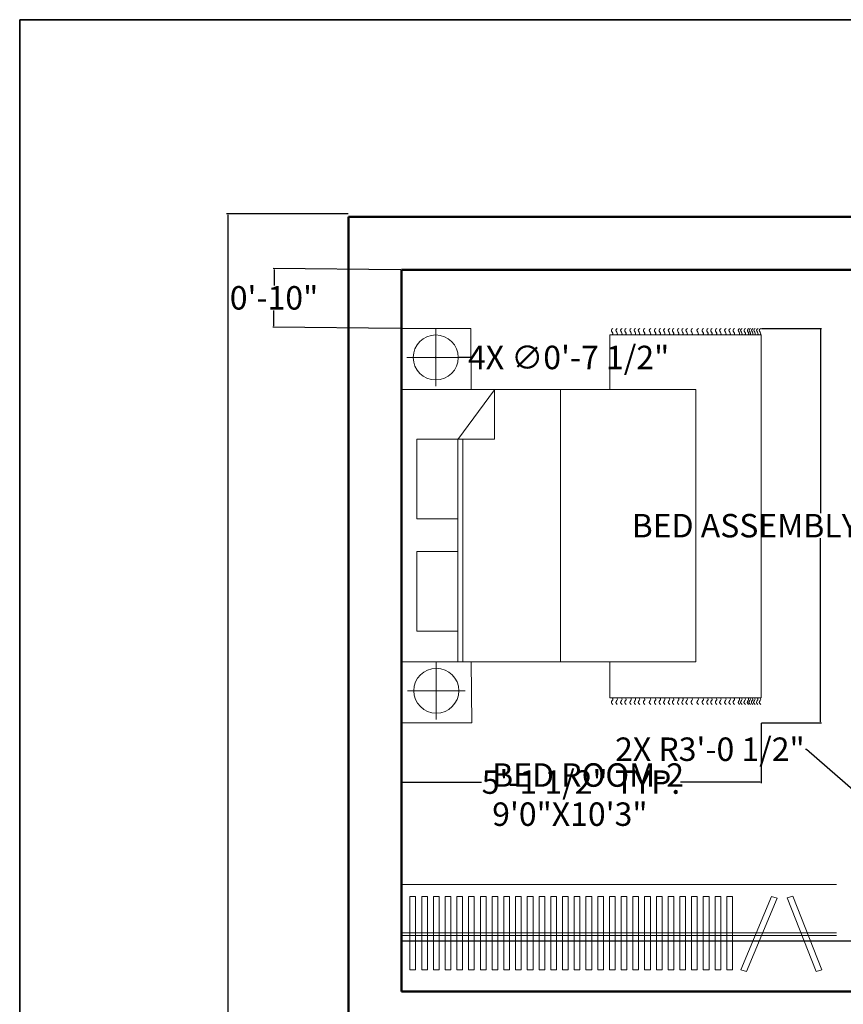
# Model space of a CAD drawing. Units: inches. Extents: x 124 to 591, y 365 to 713.
# Tile 3 of 5: x 124 to 264, y 545 to 713. Entities that reach past the tile are written whole.
import ezdxf

# ---------------------------------------------------------------- set-up
doc = ezdxf.new("R2010")
doc.units = ezdxf.units.IN
doc.header["$MEASUREMENT"] = 0
for name, color, linetype, lineweight in [('A-ANNO-DIMS', 2, 'Continuous', 18), ('A-ANNO-TTLB', 7, 'Continuous', 35), ('A-AREA-IDEN', 7, 'Continuous', 25), ('A-FLOR-CASE', 8, 'Continuous', 18), ('A-WALL', 7, 'Continuous', 50), ('furniture', 8, 'Continuous', 13)]:
    doc.layers.add(name, color=color, linetype=linetype, lineweight=lineweight)
doc.styles.get("Standard").update_dxf_attribs({"font": 'arial.ttf'})
doc.dimstyles.get("Standard").update_dxf_attribs({"dimtxt": 4, "dimasz": 0.18, "dimexe": 0.18, "dimexo": 0.0625, "dimgap": 0.09, "dimtad": 0, "dimtih": 1, "dimtoh": 1, "dimdec": 1, "dimzin": 0, "dimdsep": 46, "dimlunit": 3, "dimtxsty": 'Standard', "dimcen": 0.09, "dimclrd": 6, "dimclrt": 3, "dimadec": 0, "dimazin": 0, "dimtfac": 1, "dimtdec": 1, "dimtofl": 0, "dimtmove": 0, "dimatfit": 3, "dimfxl": 1, "dimtfillclr": 6, "dimtolj": 1, "dimtzin": 0, "dimarcsym": 0})

# ---------------------------------------------------------------- blocks, each defined once
blk = doc.blocks.new('CARPET')
at = {"layer": 'furniture'}
for p, q in [((-51.53, -98.11), (-51.53, -55.12)), ((-51.53, -55.12), (-41.27, -55.12)), ((36, -55.12), (51.55, -55.12)), ((51.55, -55.12), (51.55, -98.11)), ((51.55, -98.11), (-51.53, -98.11))]:
    blk.add_line(p, q, dxfattribs=at)
for points, knots in [([(-53.37, -55.99), (-53.22, -55.8), (-52.9, -55.41), (-52.34, -55.8), (-51.89, -56.08), (-51.65, -55.91), (-51.53, -55.83)], [0, 0, 0, 0, 0.653278, 1.290138, 1.740457, 2.114451, 2.114451, 2.114451, 2.114451]), ([(53.37, -55.99), (53.22, -55.8), (52.9, -55.41), (52.34, -55.8), (51.89, -56.08), (51.65, -55.91), (51.53, -55.83)], [0, 0, 0, 0, 0.653278, 1.290138, 1.740457, 2.114451, 2.114451, 2.114451, 2.114451]), ([(-53.37, -57.26), (-53.22, -57.07), (-52.9, -56.67), (-52.34, -57.07), (-51.89, -57.35), (-51.65, -57.17), (-51.53, -57.1)], [0, 0, 0, 0, 0.653278, 1.290138, 1.740457, 2.114451, 2.114451, 2.114451, 2.114451]), ([(-53.37, -58.59), (-53.22, -58.4), (-52.9, -58.01), (-52.34, -58.4), (-51.89, -58.68), (-51.65, -58.5), (-51.53, -58.43)], [0, 0, 0, 0, 0.653278, 1.290138, 1.740457, 2.114451, 2.114451, 2.114451, 2.114451]), ([(53.37, -57.26), (53.22, -57.07), (52.9, -56.67), (52.34, -57.07), (51.89, -57.35), (51.65, -57.17), (51.53, -57.1)], [0, 0, 0, 0, 0.653278, 1.290138, 1.740457, 2.114451, 2.114451, 2.114451, 2.114451]), ([(53.37, -58.59), (53.22, -58.4), (52.9, -58.01), (52.34, -58.4), (51.89, -58.68), (51.65, -58.5), (51.53, -58.43)], [0, 0, 0, 0, 0.653278, 1.290138, 1.740457, 2.114451, 2.114451, 2.114451, 2.114451]), ([(-53.37, -59.78), (-53.22, -59.58), (-52.9, -59.19), (-52.34, -59.58), (-51.89, -59.86), (-51.65, -59.69), (-51.53, -59.61)], [0, 0, 0, 0, 0.653278, 1.290138, 1.740457, 2.114451, 2.114451, 2.114451, 2.114451]), ([(-53.37, -61.22), (-53.22, -61.02), (-52.9, -60.63), (-52.34, -61.02), (-51.89, -61.3), (-51.65, -61.13), (-51.53, -61.05)], [0, 0, 0, 0, 0.653278, 1.290138, 1.740457, 2.114451, 2.114451, 2.114451, 2.114451]), ([(53.37, -59.78), (53.22, -59.58), (52.9, -59.19), (52.34, -59.58), (51.89, -59.86), (51.65, -59.69), (51.53, -59.61)], [0, 0, 0, 0, 0.653278, 1.290138, 1.740457, 2.114451, 2.114451, 2.114451, 2.114451]), ([(53.37, -61.22), (53.22, -61.02), (52.9, -60.63), (52.34, -61.02), (51.89, -61.3), (51.65, -61.13), (51.53, -61.05)], [0, 0, 0, 0, 0.653278, 1.290138, 1.740457, 2.114451, 2.114451, 2.114451, 2.114451]), ([(-53.37, -62.44), (-53.22, -62.25), (-52.9, -61.86), (-52.34, -62.25), (-51.89, -62.53), (-51.65, -62.36), (-51.53, -62.28)], [0, 0, 0, 0, 0.653278, 1.290138, 1.740457, 2.114451, 2.114451, 2.114451, 2.114451]), ([(-53.37, -63.63), (-53.22, -63.43), (-52.9, -63.04), (-52.34, -63.43), (-51.89, -63.72), (-51.65, -63.54), (-51.53, -63.46)], [0, 0, 0, 0, 0.653278, 1.290138, 1.740457, 2.114451, 2.114451, 2.114451, 2.114451]), ([(53.37, -62.44), (53.22, -62.25), (52.9, -61.86), (52.34, -62.25), (51.89, -62.53), (51.65, -62.36), (51.53, -62.28)], [0, 0, 0, 0, 0.653278, 1.290138, 1.740457, 2.114451, 2.114451, 2.114451, 2.114451]), ([(53.37, -63.63), (53.22, -63.43), (52.9, -63.04), (52.34, -63.43), (51.89, -63.72), (51.65, -63.54), (51.53, -63.46)], [0, 0, 0, 0, 0.653278, 1.290138, 1.740457, 2.114451, 2.114451, 2.114451, 2.114451]), ([(-53.37, -65.07), (-53.22, -64.87), (-52.9, -64.48), (-52.34, -64.87), (-51.89, -65.15), (-51.65, -64.98), (-51.53, -64.9)], [0, 0, 0, 0, 0.653278, 1.290138, 1.740457, 2.114451, 2.114451, 2.114451, 2.114451]), ([(-53.37, -66.76), (-53.22, -66.56), (-52.9, -66.17), (-52.34, -66.56), (-51.89, -66.84), (-51.65, -66.67), (-51.53, -66.59)], [0, 0, 0, 0, 0.653278, 1.290138, 1.740457, 2.114451, 2.114451, 2.114451, 2.114451]), ([(53.37, -65.07), (53.22, -64.87), (52.9, -64.48), (52.34, -64.87), (51.89, -65.15), (51.65, -64.98), (51.53, -64.9)], [0, 0, 0, 0, 0.653278, 1.290138, 1.740457, 2.114451, 2.114451, 2.114451, 2.114451]), ([(53.37, -66.76), (53.22, -66.56), (52.9, -66.17), (52.34, -66.56), (51.89, -66.84), (51.65, -66.67), (51.53, -66.59)], [0, 0, 0, 0, 0.653278, 1.290138, 1.740457, 2.114451, 2.114451, 2.114451, 2.114451]), ([(-53.37, -68.2), (-53.22, -68), (-52.9, -67.61), (-52.34, -68), (-51.89, -68.28), (-51.65, -68.11), (-51.53, -68.03)], [0, 0, 0, 0, 0.653278, 1.290138, 1.740457, 2.114451, 2.114451, 2.114451, 2.114451]), ([(-53.37, -69.53), (-53.22, -69.33), (-52.9, -68.94), (-52.34, -69.33), (-51.89, -69.61), (-51.65, -69.44), (-51.53, -69.36)], [0, 0, 0, 0, 0.653278, 1.290138, 1.740457, 2.114451, 2.114451, 2.114451, 2.114451]), ([(53.37, -68.2), (53.22, -68), (52.9, -67.61), (52.34, -68), (51.89, -68.28), (51.65, -68.11), (51.53, -68.03)], [0, 0, 0, 0, 0.653278, 1.290138, 1.740457, 2.114451, 2.114451, 2.114451, 2.114451]), ([(53.37, -69.53), (53.22, -69.33), (52.9, -68.94), (52.34, -69.33), (51.89, -69.61), (51.65, -69.44), (51.53, -69.36)], [0, 0, 0, 0, 0.653278, 1.290138, 1.740457, 2.114451, 2.114451, 2.114451, 2.114451]), ([(-53.37, -70.79), (-53.22, -70.6), (-52.9, -70.21), (-52.34, -70.6), (-51.89, -70.88), (-51.65, -70.7), (-51.53, -70.63)], [0, 0, 0, 0, 0.653278, 1.290138, 1.740457, 2.114451, 2.114451, 2.114451, 2.114451]), ([(-53.37, -72.12), (-53.22, -71.93), (-52.9, -71.54), (-52.34, -71.93), (-51.89, -72.21), (-51.65, -72.04), (-51.53, -71.96)], [0, 0, 0, 0, 0.653278, 1.290138, 1.740457, 2.114451, 2.114451, 2.114451, 2.114451]), ([(53.37, -70.79), (53.22, -70.6), (52.9, -70.21), (52.34, -70.6), (51.89, -70.88), (51.65, -70.7), (51.53, -70.63)], [0, 0, 0, 0, 0.653278, 1.290138, 1.740457, 2.114451, 2.114451, 2.114451, 2.114451]), ([(53.37, -72.12), (53.22, -71.93), (52.9, -71.54), (52.34, -71.93), (51.89, -72.21), (51.65, -72.04), (51.53, -71.96)], [0, 0, 0, 0, 0.653278, 1.290138, 1.740457, 2.114451, 2.114451, 2.114451, 2.114451]), ([(-53.37, -73.31), (-53.22, -73.11), (-52.9, -72.72), (-52.34, -73.11), (-51.89, -73.4), (-51.65, -73.22), (-51.53, -73.14)], [0, 0, 0, 0, 0.653278, 1.290138, 1.740457, 2.114451, 2.114451, 2.114451, 2.114451]), ([(-53.37, -74.75), (-53.22, -74.55), (-52.9, -74.16), (-52.34, -74.55), (-51.89, -74.83), (-51.65, -74.66), (-51.53, -74.58)], [0, 0, 0, 0, 0.653278, 1.290138, 1.740457, 2.114451, 2.114451, 2.114451, 2.114451]), ([(53.37, -73.31), (53.22, -73.11), (52.9, -72.72), (52.34, -73.11), (51.89, -73.4), (51.65, -73.22), (51.53, -73.14)], [0, 0, 0, 0, 0.653278, 1.290138, 1.740457, 2.114451, 2.114451, 2.114451, 2.114451]), ([(53.37, -74.75), (53.22, -74.55), (52.9, -74.16), (52.34, -74.55), (51.89, -74.83), (51.65, -74.66), (51.53, -74.58)], [0, 0, 0, 0, 0.653278, 1.290138, 1.740457, 2.114451, 2.114451, 2.114451, 2.114451]), ([(-53.37, -75.98), (-53.22, -75.78), (-52.9, -75.39), (-52.34, -75.78), (-51.89, -76.06), (-51.65, -75.89), (-51.53, -75.81)], [0, 0, 0, 0, 0.653278, 1.290138, 1.740457, 2.114451, 2.114451, 2.114451, 2.114451]), ([(-53.37, -77.16), (-53.22, -76.96), (-52.9, -76.57), (-52.34, -76.96), (-51.89, -77.25), (-51.65, -77.07), (-51.53, -76.99)], [0, 0, 0, 0, 0.653278, 1.290138, 1.740457, 2.114451, 2.114451, 2.114451, 2.114451]), ([(-53.37, -78.6), (-53.22, -78.4), (-52.9, -78.01), (-52.34, -78.4), (-51.89, -78.68), (-51.65, -78.51), (-51.53, -78.43)], [0, 0, 0, 0, 0.653278, 1.290138, 1.740457, 2.114451, 2.114451, 2.114451, 2.114451]), ([(53.37, -75.98), (53.22, -75.78), (52.9, -75.39), (52.34, -75.78), (51.89, -76.06), (51.65, -75.89), (51.53, -75.81)], [0, 0, 0, 0, 0.653278, 1.290138, 1.740457, 2.114451, 2.114451, 2.114451, 2.114451]), ([(53.37, -77.16), (53.22, -76.96), (52.9, -76.57), (52.34, -76.96), (51.89, -77.25), (51.65, -77.07), (51.53, -76.99)], [0, 0, 0, 0, 0.653278, 1.290138, 1.740457, 2.114451, 2.114451, 2.114451, 2.114451]), ([(53.37, -78.6), (53.22, -78.4), (52.9, -78.01), (52.34, -78.4), (51.89, -78.68), (51.65, -78.51), (51.53, -78.43)], [0, 0, 0, 0, 0.653278, 1.290138, 1.740457, 2.114451, 2.114451, 2.114451, 2.114451]), ([(-53.37, -80.29), (-53.22, -80.09), (-52.9, -79.7), (-52.34, -80.09), (-51.89, -80.37), (-51.65, -80.2), (-51.53, -80.12)], [0, 0, 0, 0, 0.653278, 1.290138, 1.740457, 2.114451, 2.114451, 2.114451, 2.114451]), ([(53.37, -80.29), (53.22, -80.09), (52.9, -79.7), (52.34, -80.09), (51.89, -80.37), (51.65, -80.2), (51.53, -80.12)], [0, 0, 0, 0, 0.653278, 1.290138, 1.740457, 2.114451, 2.114451, 2.114451, 2.114451]), ([(-53.37, -81.73), (-53.22, -81.53), (-52.9, -81.14), (-52.34, -81.53), (-51.89, -81.81), (-51.65, -81.64), (-51.53, -81.56)], [0, 0, 0, 0, 0.653278, 1.290138, 1.740457, 2.114451, 2.114451, 2.114451, 2.114451]), ([(-53.37, -83.06), (-53.22, -82.86), (-52.9, -82.47), (-52.34, -82.86), (-51.89, -83.14), (-51.65, -82.97), (-51.53, -82.89)], [0, 0, 0, 0, 0.653278, 1.290138, 1.740457, 2.114451, 2.114451, 2.114451, 2.114451]), ([(-53.37, -84.18), (-53.22, -83.99), (-52.9, -83.6), (-52.34, -83.99), (-51.89, -84.27), (-51.65, -84.09), (-51.53, -84.02)], [0, 0, 0, 0, 0.653278, 1.290138, 1.740457, 2.114451, 2.114451, 2.114451, 2.114451]), ([(53.37, -81.73), (53.22, -81.53), (52.9, -81.14), (52.34, -81.53), (51.89, -81.81), (51.65, -81.64), (51.53, -81.56)], [0, 0, 0, 0, 0.653278, 1.290138, 1.740457, 2.114451, 2.114451, 2.114451, 2.114451]), ([(53.37, -83.06), (53.22, -82.86), (52.9, -82.47), (52.34, -82.86), (51.89, -83.14), (51.65, -82.97), (51.53, -82.89)], [0, 0, 0, 0, 0.653278, 1.290138, 1.740457, 2.114451, 2.114451, 2.114451, 2.114451]), ([(53.37, -84.18), (53.22, -83.99), (52.9, -83.6), (52.34, -83.99), (51.89, -84.27), (51.65, -84.09), (51.53, -84.02)], [0, 0, 0, 0, 0.653278, 1.290138, 1.740457, 2.114451, 2.114451, 2.114451, 2.114451]), ([(-53.37, -85.51), (-53.22, -85.32), (-52.9, -84.93), (-52.34, -85.32), (-51.89, -85.6), (-51.65, -85.42), (-51.53, -85.35)], [0, 0, 0, 0, 0.653278, 1.290138, 1.740457, 2.114451, 2.114451, 2.114451, 2.114451]), ([(-53.37, -86.7), (-53.22, -86.5), (-52.9, -86.11), (-52.34, -86.5), (-51.89, -86.78), (-51.65, -86.61), (-51.53, -86.53)], [0, 0, 0, 0, 0.653278, 1.290138, 1.740457, 2.114451, 2.114451, 2.114451, 2.114451]), ([(53.37, -85.51), (53.22, -85.32), (52.9, -84.93), (52.34, -85.32), (51.89, -85.6), (51.65, -85.42), (51.53, -85.35)], [0, 0, 0, 0, 0.653278, 1.290138, 1.740457, 2.114451, 2.114451, 2.114451, 2.114451]), ([(53.37, -86.7), (53.22, -86.5), (52.9, -86.11), (52.34, -86.5), (51.89, -86.78), (51.65, -86.61), (51.53, -86.53)], [0, 0, 0, 0, 0.653278, 1.290138, 1.740457, 2.114451, 2.114451, 2.114451, 2.114451]), ([(-53.37, -88.14), (-53.22, -87.94), (-52.9, -87.55), (-52.34, -87.94), (-51.89, -88.22), (-51.65, -88.05), (-51.53, -87.97)], [0, 0, 0, 0, 0.653278, 1.290138, 1.740457, 2.114451, 2.114451, 2.114451, 2.114451]), ([(-53.37, -89.36), (-53.22, -89.17), (-52.9, -88.78), (-52.34, -89.17), (-51.89, -89.45), (-51.65, -89.28), (-51.53, -89.2)], [0, 0, 0, 0, 0.653278, 1.290138, 1.740457, 2.114451, 2.114451, 2.114451, 2.114451]), ([(53.37, -88.14), (53.22, -87.94), (52.9, -87.55), (52.34, -87.94), (51.89, -88.22), (51.65, -88.05), (51.53, -87.97)], [0, 0, 0, 0, 0.653278, 1.290138, 1.740457, 2.114451, 2.114451, 2.114451, 2.114451]), ([(53.37, -89.36), (53.22, -89.17), (52.9, -88.78), (52.34, -89.17), (51.89, -89.45), (51.65, -89.28), (51.53, -89.2)], [0, 0, 0, 0, 0.653278, 1.290138, 1.740457, 2.114451, 2.114451, 2.114451, 2.114451]), ([(-53.37, -90.55), (-53.22, -90.35), (-52.9, -89.96), (-52.34, -90.35), (-51.89, -90.64), (-51.65, -90.46), (-51.53, -90.38)], [0, 0, 0, 0, 0.653278, 1.290138, 1.740457, 2.114451, 2.114451, 2.114451, 2.114451]), ([(-53.37, -91.99), (-53.22, -91.79), (-52.9, -91.4), (-52.34, -91.79), (-51.89, -92.07), (-51.65, -91.9), (-51.53, -91.82)], [0, 0, 0, 0, 0.653278, 1.290138, 1.740457, 2.114451, 2.114451, 2.114451, 2.114451]), ([(-53.37, -92.69), (-53.22, -92.48), (-52.9, -92.08), (-52.35, -92.49), (-51.89, -92.77), (-51.65, -92.6), (-51.53, -92.52)], [0, 0, 0, 0, 0.663904, 1.307406, 1.757725, 2.131719, 2.131719, 2.131719, 2.131719]), ([(53.37, -90.55), (53.22, -90.35), (52.9, -89.96), (52.34, -90.35), (51.9, -90.63), (51.66, -90.47), (51.55, -90.4)], [0, 0, 0, 0, 0.653278, 1.290138, 1.740457, 2.0926, 2.0926, 2.0926, 2.0926]), ([(53.37, -91.99), (53.22, -91.79), (52.9, -91.4), (52.34, -91.79), (51.9, -92.07), (51.66, -91.91), (51.55, -91.83)], [0, 0, 0, 0, 0.653278, 1.290138, 1.740457, 2.0926, 2.0926, 2.0926, 2.0926]), ([(53.37, -92.69), (53.22, -92.49), (52.9, -92.09), (52.34, -92.49), (51.9, -92.77), (51.66, -92.61), (51.55, -92.53)], [0, 0, 0, 0, 0.656792, 1.295826, 1.746145, 2.098292, 2.098292, 2.098292, 2.098292]), ([(-53.37, -93.61), (-53.22, -93.42), (-52.9, -93.03), (-52.34, -93.42), (-51.89, -93.7), (-51.65, -93.52), (-51.53, -93.45)], [0, 0, 0, 0, 0.653278, 1.290138, 1.740457, 2.114451, 2.114451, 2.114451, 2.114451]), ([(-53.37, -94.55), (-53.22, -94.35), (-52.9, -93.96), (-52.34, -94.35), (-51.89, -94.63), (-51.65, -94.46), (-51.53, -94.38)], [0, 0, 0, 0, 0.653278, 1.290138, 1.740457, 2.114451, 2.114451, 2.114451, 2.114451]), ([(-53.37, -95.05), (-53.22, -94.85), (-52.9, -94.46), (-52.34, -94.85), (-51.89, -95.14), (-51.65, -94.96), (-51.53, -94.88)], [0, 0, 0, 0, 0.653278, 1.290138, 1.740457, 2.114451, 2.114451, 2.114451, 2.114451]), ([(53.37, -93.66), (53.22, -93.46), (52.9, -93.07), (52.34, -93.46), (51.9, -93.74), (51.66, -93.58), (51.55, -93.5)], [0, 0, 0, 0, 0.653278, 1.290138, 1.740457, 2.0926, 2.0926, 2.0926, 2.0926]), ([(53.37, -94.59), (53.22, -94.4), (52.9, -94.01), (52.34, -94.4), (51.9, -94.68), (51.66, -94.51), (51.55, -94.44)], [0, 0, 0, 0, 0.653278, 1.290138, 1.740457, 2.0926, 2.0926, 2.0926, 2.0926]), ([(53.37, -95.1), (53.22, -94.9), (52.9, -94.51), (52.34, -94.9), (51.9, -95.18), (51.66, -95.02), (51.55, -94.94)], [0, 0, 0, 0, 0.653278, 1.290138, 1.740457, 2.0926, 2.0926, 2.0926, 2.0926]), ([(-53.37, -95.73), (-53.22, -95.54), (-52.9, -95.15), (-52.34, -95.54), (-51.89, -95.82), (-51.65, -95.65), (-51.53, -95.57)], [0, 0, 0, 0, 0.653278, 1.290138, 1.740457, 2.114451, 2.114451, 2.114451, 2.114451]), ([(-53.37, -96.38), (-53.22, -96.18), (-52.9, -95.79), (-52.34, -96.18), (-51.89, -96.47), (-51.65, -96.29), (-51.53, -96.21)], [0, 0, 0, 0, 0.653278, 1.290138, 1.740457, 2.114451, 2.114451, 2.114451, 2.114451]), ([(-53.37, -97.17), (-53.22, -96.98), (-52.9, -96.59), (-52.34, -96.98), (-51.89, -97.26), (-51.65, -97.08), (-51.53, -97.01)], [0, 0, 0, 0, 0.653278, 1.290138, 1.740457, 2.114451, 2.114451, 2.114451, 2.114451]), ([(-53.37, -97.99), (-53.22, -97.79), (-52.9, -97.4), (-52.34, -97.79), (-51.89, -98.08), (-51.65, -97.9), (-51.53, -97.82)], [0, 0, 0, 0, 0.653278, 1.290138, 1.740457, 2.114451, 2.114451, 2.114451, 2.114451]), ([(53.37, -95.78), (53.22, -95.58), (52.9, -95.19), (52.34, -95.58), (51.89, -95.86), (51.65, -95.69), (51.53, -95.61)], [0, 0, 0, 0, 0.653278, 1.290138, 1.740457, 2.114451, 2.114451, 2.114451, 2.114451]), ([(53.37, -96.43), (53.22, -96.23), (52.9, -95.84), (52.34, -96.23), (51.89, -96.51), (51.65, -96.34), (51.53, -96.26)], [0, 0, 0, 0, 0.653278, 1.290138, 1.740457, 2.114451, 2.114451, 2.114451, 2.114451]), ([(53.37, -97.22), (53.22, -97.02), (52.9, -96.63), (52.34, -97.02), (51.89, -97.3), (51.65, -97.13), (51.53, -97.05)], [0, 0, 0, 0, 0.653278, 1.290138, 1.740457, 2.114451, 2.114451, 2.114451, 2.114451]), ([(53.37, -97.99), (53.22, -97.79), (52.9, -97.4), (52.34, -97.79), (51.89, -98.08), (51.65, -97.9), (51.53, -97.82)], [0, 0, 0, 0, 0.653278, 1.290138, 1.740457, 2.114451, 2.114451, 2.114451, 2.114451])]:
    blk.add_open_spline(points, degree=3, knots=knots, dxfattribs=at)
blk = doc.blocks.new('A$C58D270C6')
at = {"layer": 'furniture'}
for p, q in [((9.09, 124.13), (9.09, 108.87)), ((1.46, 116.5), (16.73, 116.5)), ((14.97, 94.84), (24.62, 107.92)), ((24.62, 94.93), (24.62, 107.92)), ((42.08, 108), (42.08, 36)), ((14.97, 94.93), (24.62, 94.93)), ((14.97, 94.84), (14.97, 36)), ((16.22, 94.93), (16.22, 36)), ((9.25, 36), (9.25, 20.74)), ((1.62, 28.37), (16.88, 28.37))]:
    blk.add_line(p, q, dxfattribs=at)
for points in [[(18.5, 108), (18.34, 124.13), (-0.16, 124.13), (0, 108)], [(0, 108), (77.91, 108), (77.91, 36), (0, 36)], [(4.09, 94.93), (14.97, 94.93), (14.97, 73.83), (4.09, 73.83)], [(4.09, 65.23), (14.97, 65.23), (14.97, 44.13), (4.09, 44.13)], [(18.65, 19.87), (18.5, 36), (0, 36), (0.16, 19.87)]]:
    blk.add_lwpolyline(points, close=True, dxfattribs=at)
for centre in [(9.09, 116.5), (9.25, 28.37)]:
    blk.add_circle(centre, 5.95, dxfattribs=at)
at = {"layer": 'furniture', "xscale": 0.9312884925094044, "yscale": 0.9312884925094044, "zscale": 0.9312884925094044, "rotation": 90}
blk.add_blockref('CARPET', (3.79, 74.47), dxfattribs=at)
blk = doc.blocks.new('*D20')
at = {"layer": 'A-ANNO-DIMS', "color": 0, "lineweight": -2, "transparency": 16777216}
for p, q in [((180.08, 679.59), (159.36, 679.59)), ((159.54, 679.41), (159.54, 536.98)), ((159.54, 390.27), (159.54, 532.71)), ((180.08, 390.09), (159.36, 390.09))]:
    blk.add_line(p, q, dxfattribs=at)
at = {"layer": 'A-ANNO-DIMS', "color": 0, "transparency": 16777216}
for points in [[(159.51, 679.41), (159.57, 679.41), (159.54, 679.59)], [(159.51, 390.27), (159.57, 390.27), (159.54, 390.09)]]:
    blk.add_solid(points, dxfattribs=at)
at = {"layer": 'Defpoints', "color": 0, "transparency": 16777216}
for p in [(159.54, 679.59), (180.14, 679.59), (180.14, 390.09)]:
    blk.add_point(p, dxfattribs=at)
at = {"layer": 'A-ANNO-DIMS', "color": 0, "transparency": 16777216, "insert": (159.54, 534.84), "char_height": 4, "attachment_point": 5}
blk.add_mtext('\\A1;24\'-1.5"', dxfattribs=at)
blk = doc.blocks.new('*D24')
at = {"layer": 'A-ANNO-DIMS', "color": 0, "lineweight": -2, "transparency": 16777216}
for p, q in [((189.14, 547.36), (189.14, 555.91)), ((189.32, 555.73), (278.29, 555.73)), ((385.46, 555.73), (296.49, 555.73)), ((385.64, 547.15), (385.64, 555.91))]:
    blk.add_line(p, q, dxfattribs=at)
at = {"layer": 'A-ANNO-DIMS', "color": 0, "transparency": 16777216}
for points in [[(189.32, 555.76), (189.32, 555.7), (189.14, 555.73)], [(385.46, 555.76), (385.46, 555.7), (385.64, 555.73)]]:
    blk.add_solid(points, dxfattribs=at)
at = {"layer": 'Defpoints', "color": 0, "transparency": 16777216}
for p in [(385.64, 555.73), (189.14, 547.3), (385.64, 547.09)]:
    blk.add_point(p, dxfattribs=at)
at = {"layer": 'A-ANNO-DIMS', "color": 0, "transparency": 16777216, "insert": (287.39, 555.73), "char_height": 4, "attachment_point": 5}
blk.add_mtext('\\A1;16\'-4.5"', dxfattribs=at)
blk = doc.blocks.new('WARDROBE-HANGING-RAIL')
for p, q in [((0, 18), (74.16, 18)), ((0, 0), (0, 18)), ((0, 9.79), (74.16, 9.79)), ((0, 9.29), (74.16, 9.29))]:
    blk.add_line(p, q)
for points in [[(1.47, 3.44), (1.47, 15.95), (2.44, 15.95), (2.44, 3.44)], [(3.47, 3.44), (3.47, 15.95), (4.44, 15.95), (4.44, 3.44)], [(5.47, 3.44), (5.47, 15.95), (6.44, 15.95), (6.44, 3.44)], [(7.47, 3.44), (7.47, 15.95), (8.44, 15.95), (8.44, 3.44)], [(7.47, 3.44), (7.47, 15.95), (8.44, 15.95), (8.44, 3.44)], [(9.47, 3.44), (9.47, 15.95), (10.44, 15.95), (10.44, 3.44)], [(11.47, 3.44), (11.47, 15.95), (12.44, 15.95), (12.44, 3.44)], [(13.47, 3.44), (13.47, 15.95), (14.44, 15.95), (14.44, 3.44)], [(15.47, 3.44), (15.47, 15.95), (16.44, 15.95), (16.44, 3.44)], [(17.47, 3.44), (17.47, 15.95), (18.44, 15.95), (18.44, 3.44)], [(19.47, 3.44), (19.47, 15.95), (20.44, 15.95), (20.44, 3.44)], [(19.47, 3.44), (19.47, 15.95), (20.44, 15.95), (20.44, 3.44)], [(21.47, 3.44), (21.47, 15.95), (22.44, 15.95), (22.44, 3.44)], [(23.47, 3.44), (23.47, 15.95), (24.44, 15.95), (24.44, 3.44)], [(25.47, 3.44), (25.47, 15.95), (26.44, 15.95), (26.44, 3.44)], [(27.47, 3.44), (27.47, 15.95), (28.44, 15.95), (28.44, 3.44)], [(29.47, 3.44), (29.47, 15.95), (30.44, 15.95), (30.44, 3.44)], [(31.47, 3.44), (31.47, 15.95), (32.44, 15.95), (32.44, 3.44)], [(31.47, 3.44), (31.47, 15.95), (32.44, 15.95), (32.44, 3.44)], [(33.47, 3.44), (33.47, 15.95), (34.44, 15.95), (34.44, 3.44)], [(35.47, 3.44), (35.47, 15.95), (36.44, 15.95), (36.44, 3.44)], [(37.47, 3.44), (37.47, 15.95), (38.44, 15.95), (38.44, 3.44)], [(39.47, 3.44), (39.47, 15.95), (40.44, 15.95), (40.44, 3.44)], [(41.47, 3.44), (41.47, 15.95), (42.44, 15.95), (42.44, 3.44)], [(43.47, 3.44), (43.47, 15.95), (44.44, 15.95), (44.44, 3.44)], [(43.47, 3.44), (43.47, 15.95), (44.44, 15.95), (44.44, 3.44)], [(45.47, 3.44), (45.47, 15.95), (46.44, 15.95), (46.44, 3.44)], [(47.47, 3.44), (47.47, 15.95), (48.44, 15.95), (48.44, 3.44)], [(49.47, 3.44), (49.47, 15.95), (50.44, 15.95), (50.44, 3.44)], [(51.47, 3.44), (51.47, 15.95), (52.44, 15.95), (52.44, 3.44)], [(53.47, 3.44), (53.47, 15.95), (54.44, 15.95), (54.44, 3.44)], [(55.47, 3.44), (55.47, 15.95), (56.44, 15.95), (56.44, 3.44)], [(57.87, 3.44), (58.83, 3.15), (64.04, 15.66), (63.08, 15.95)], [(70.7, 3.17), (71.66, 3.45), (66.73, 16.04), (65.77, 15.76)]]:
    blk.add_lwpolyline(points, close=True)
blk = doc.blocks.new('*D28')
at = {"layer": 'A-ANNO-DIMS', "color": 0, "lineweight": -2, "transparency": 16777216}
for p, q in [((250.53, 660.08), (260.74, 660.08)), ((250.53, 592.85), (260.74, 592.85))]:
    blk.add_line(p, q, dxfattribs=at)
at = {"layer": 'A-ANNO-DIMS', "color": 6, "lineweight": -2, "transparency": 16777216}
for p, q in [((260.56, 659.9), (260.56, 628.62)), ((260.56, 593.03), (260.56, 624.31))]:
    blk.add_line(p, q, dxfattribs=at)
at = {"layer": 'A-ANNO-DIMS', "color": 6, "transparency": 16777216}
for points in [[(260.53, 659.9), (260.59, 659.9), (260.56, 660.08)], [(260.53, 593.03), (260.59, 593.03), (260.56, 592.85)]]:
    blk.add_solid(points, dxfattribs=at)
at = {"layer": 'Defpoints', "color": 0, "transparency": 16777216}
for p in [(250.47, 660.08), (260.56, 660.08), (250.47, 592.85)]:
    blk.add_point(p, dxfattribs=at)
at = {"layer": 'A-ANNO-DIMS', "color": 3, "transparency": 16777216, "insert": (260.56, 626.46), "char_height": 4, "attachment_point": 5}
blk.add_mtext('\\A1;BED ASSEMBLY 5\'-7" TYP.', dxfattribs=at)
blk = doc.blocks.new('*D29')
at = {"layer": 'A-ANNO-DIMS', "color": 0, "lineweight": -2, "transparency": 16777216}
for p, q in [((189.04, 592.79), (189.04, 582.58)), ((250.47, 592.79), (250.47, 582.58))]:
    blk.add_line(p, q, dxfattribs=at)
at = {"layer": 'A-ANNO-DIMS', "color": 6, "lineweight": -2, "transparency": 16777216}
for p, q in [((189.22, 582.76), (202.81, 582.76)), ((250.29, 582.76), (236.7, 582.76))]:
    blk.add_line(p, q, dxfattribs=at)
at = {"layer": 'A-ANNO-DIMS', "color": 6, "transparency": 16777216}
for points in [[(189.22, 582.79), (189.22, 582.73), (189.04, 582.76)], [(250.29, 582.79), (250.29, 582.73), (250.47, 582.76)]]:
    blk.add_solid(points, dxfattribs=at)
at = {"layer": 'Defpoints', "color": 0, "transparency": 16777216}
for p in [(189.04, 592.85), (250.47, 592.85), (250.47, 582.76)]:
    blk.add_point(p, dxfattribs=at)
at = {"layer": 'A-ANNO-DIMS', "color": 3, "transparency": 16777216, "insert": (219.75, 582.76), "char_height": 4, "attachment_point": 5}
blk.add_mtext('\\A1;5\'-1 1/2" TYP.', dxfattribs=at)
blk = doc.blocks.new('*D65')
at = {"layer": 'A-ANNO-DIMS', "color": 0, "lineweight": -2, "transparency": 16777216}
for p, q in [((189.08, 670.09), (167.31, 670.31)), ((188.98, 660.05), (167.21, 660.27))]:
    blk.add_line(p, q, dxfattribs=at)
at = {"layer": 'A-ANNO-DIMS', "color": 6, "lineweight": -2, "transparency": 16777216}
for p, q in [((167.49, 670.13), (167.46, 667.42)), ((167.39, 660.44), (167.42, 663.15))]:
    blk.add_line(p, q, dxfattribs=at)
at = {"layer": 'A-ANNO-DIMS', "color": 6, "transparency": 16777216}
for points in [[(167.46, 670.13), (167.52, 670.13), (167.49, 670.31)], [(167.36, 660.44), (167.42, 660.44), (167.39, 660.26)]]:
    blk.add_solid(points, dxfattribs=at)
at = {"layer": 'Defpoints', "color": 0, "transparency": 16777216}
for p in [(167.49, 670.31), (189.14, 670.09), (189.04, 660.05)]:
    blk.add_point(p, dxfattribs=at)
at = {"layer": 'A-ANNO-DIMS', "color": 3, "transparency": 16777216, "insert": (167.44, 665.29), "char_height": 4, "attachment_point": 5}
blk.add_mtext('\\A1;0\'-10"', dxfattribs=at)
blk = doc.blocks.new('*D68')
at = {"layer": 'A-ANNO-DIMS', "color": 6, "lineweight": -2, "transparency": 16777216}
for p, q in [((258.04, 588.36), (258.22, 588.36)), ((258.22, 588.36), (274.49, 574.13))]:
    blk.add_line(p, q, dxfattribs=at)
at = {"layer": 'A-ANNO-DIMS', "color": 0, "lineweight": -2, "transparency": 16777216}
for p, q in [((301.87, 550.09), (302.05, 550.09)), ((301.96, 550), (301.96, 550.18))]:
    blk.add_line(p, q, dxfattribs=at)
at = {"layer": 'A-ANNO-DIMS', "color": 6, "transparency": 16777216}
blk.add_solid([(274.51, 574.15), (274.47, 574.11), (274.62, 574.01)], dxfattribs=at)
at = {"layer": 'Defpoints', "color": 0, "transparency": 16777216}
for p in [(274.62, 574.01), (301.96, 550.09)]:
    blk.add_point(p, dxfattribs=at)
at = {"layer": 'A-ANNO-DIMS', "color": 3, "transparency": 16777216, "insert": (241.73, 588.36), "char_height": 4, "attachment_point": 5}
blk.add_mtext('\\A1;2X R3\'-0 1/2"', dxfattribs=at)
blk = doc.blocks.new('*D72')
at = {"layer": 'A-ANNO-DIMS', "color": 0, "lineweight": -2, "transparency": 16777216}
for p, q in [((194.91, 655.13), (195.09, 655.13)), ((195, 655.04), (195, 655.22))]:
    blk.add_line(p, q, dxfattribs=at)
at = {"layer": 'A-ANNO-DIMS', "color": 6, "lineweight": -2, "transparency": 16777216}
blk.add_line((201.14, 655.13), (199.02, 655.13), dxfattribs=at)
at = {"layer": 'A-ANNO-DIMS', "color": 6, "transparency": 16777216}
blk.add_solid([(199.02, 655.16), (199.02, 655.1), (198.84, 655.13)], dxfattribs=at)
at = {"layer": 'Defpoints', "color": 0, "transparency": 16777216}
for p in [(191.16, 655.13), (198.84, 655.13)]:
    blk.add_point(p, dxfattribs=at)
at = {"layer": 'A-ANNO-DIMS', "color": 3, "transparency": 16777216, "insert": (217.65, 655.13), "char_height": 4, "attachment_point": 5}
blk.add_mtext('\\A1;4X ∅0\'-7 1/2"', dxfattribs=at)

msp = doc.modelspace()

# ---------------------------------------------------------------- linework, layer by layer
at = {"layer": 'A-ANNO-TTLB'}
msp.add_lwpolyline([(124.09, 712.7), (590.57, 712.7), (590.57, 365.95), (124.09, 365.95)], close=True, dxfattribs=at)
msp.add_lwpolyline([(124.09, 712.7), (590.57, 712.7), (590.57, 365.95), (124.09, 365.95)], close=True, dxfattribs=at)
at = {"layer": 'A-WALL'}
for p, q in [((180.14, 679.09), (562.14, 679.09)), ((180.14, 679.09), (180.14, 389.59)), ((189.14, 670.09), (297.14, 670.09)), ((189.14, 670.09), (189.14, 547.09)), ((189.14, 547.09), (297.14, 547.09))]:
    msp.add_line(p, q, dxfattribs=at)

# ---------------------------------------------------------------- block references
at = {"layer": 'A-FLOR-CASE'}
msp.add_blockref('WARDROBE-HANGING-RAIL', (189.14, 547.3), dxfattribs=at)
at = {"layer": 'furniture', "xscale": 0.6445294581626225, "yscale": 0.6445294581626225, "zscale": 0.6445294581626225}
msp.add_blockref('A$C58D270C6', (189.14, 580.04), dxfattribs=at)

# ---------------------------------------------------------------- texts
at = {"layer": 'A-AREA-IDEN', "insert": (204.62, 585.96), "char_height": 4, "attachment_point": 1}
msp.add_mtext_dynamic_manual_height_columns('BED ROOM-2\\P9\'0"X10\'3"', width=64.1939, gutter_width=1, heights=[0], dxfattribs=at)

# ---------------------------------------------------------------- dimensions: what is measured, and where the dimension line sits
at = {"layer": 'A-ANNO-DIMS'}
for base, p1, p2, angle, override, picture, middle in [((159.54, 679.59), (180.14, 390.09), (180.14, 679.59), 90, {"dimclrd": 0, "dimclre": 0, "dimclrt": 0}, '*D20', (159.54, 534.84)), ((167.49, 670.31), (189.04, 660.05), (189.14, 670.09), 89.4281, {"dimdec": 1, "dimlfac": 1, "dimrnd": 0, "dimzin": 1, "dimdsep": 46, "dimlunit": 4, "dimfrac": 2}, '*D65', (167.44, 665.29))]:
    dim = msp.add_linear_dim(base=base, p1=p1, p2=p2, angle=angle, dimstyle='Standard', override=override, dxfattribs=at)
    dim.commit()
    dim.dimension.update_dxf_attribs({"geometry": picture, "text_midpoint": middle})
dim = msp.add_diameter_dim_2p(p1=(191.16, 655.13), p2=(198.84, 655.13), text='4X <>', dimstyle='Standard', override={"dimdec": 1, "dimlfac": 1, "dimrnd": 0, "dimzin": 1, "dimdsep": 46, "dimlunit": 4, "dimfrac": 2}, dxfattribs=at)
dim.commit()
dim.dimension.update_dxf_attribs({"geometry": '*D72', "text_midpoint": (201.14, 655.13), "dimtype": 163})
dim = msp.add_linear_dim(base=(260.56, 660.08), p1=(250.47, 592.85), p2=(250.47, 660.08), angle=90, text='BED ASSEMBLY <> TYP.', dimstyle='Standard', override={"dimdec": 1, "dimlfac": 1, "dimrnd": 0, "dimzin": 1, "dimdsep": 46, "dimlunit": 4, "dimfrac": 2}, dxfattribs=at)
dim.commit()
dim.dimension.update_dxf_attribs({"geometry": '*D28', "text_midpoint": (260.56, 626.46)})
dim = msp.add_radius_dim(center=(301.96, 550.09), mpoint=(274.62, 574.01), text='2X <>', dimstyle='Standard', override={"dimdec": 1, "dimlfac": 1, "dimrnd": 0, "dimzin": 1, "dimdsep": 46, "dimlunit": 4, "dimfrac": 2}, dxfattribs=at)
dim.commit()
dim.dimension.update_dxf_attribs({"geometry": '*D68', "text_midpoint": (241.73, 588.36), "dimtype": 164})
dim = msp.add_linear_dim(base=(250.47, 582.76), p1=(189.04, 592.85), p2=(250.47, 592.85), text='<> TYP.', dimstyle='Standard', override={"dimdec": 1, "dimlfac": 1, "dimrnd": 0, "dimzin": 1, "dimdsep": 46, "dimlunit": 4, "dimfrac": 2}, dxfattribs=at)
dim.commit()
dim.dimension.update_dxf_attribs({"geometry": '*D29', "text_midpoint": (219.75, 582.76)})
dim = msp.add_linear_dim(base=(385.64, 555.73), p1=(189.14, 547.3), p2=(385.64, 547.09), dimstyle='Standard', override={"dimclrd": 0, "dimclre": 0, "dimclrt": 0}, dxfattribs=at)
dim.commit()
dim.dimension.update_dxf_attribs({"geometry": '*D24', "text_midpoint": (287.39, 555.73)})

doc.saveas('drawing.dxf')
